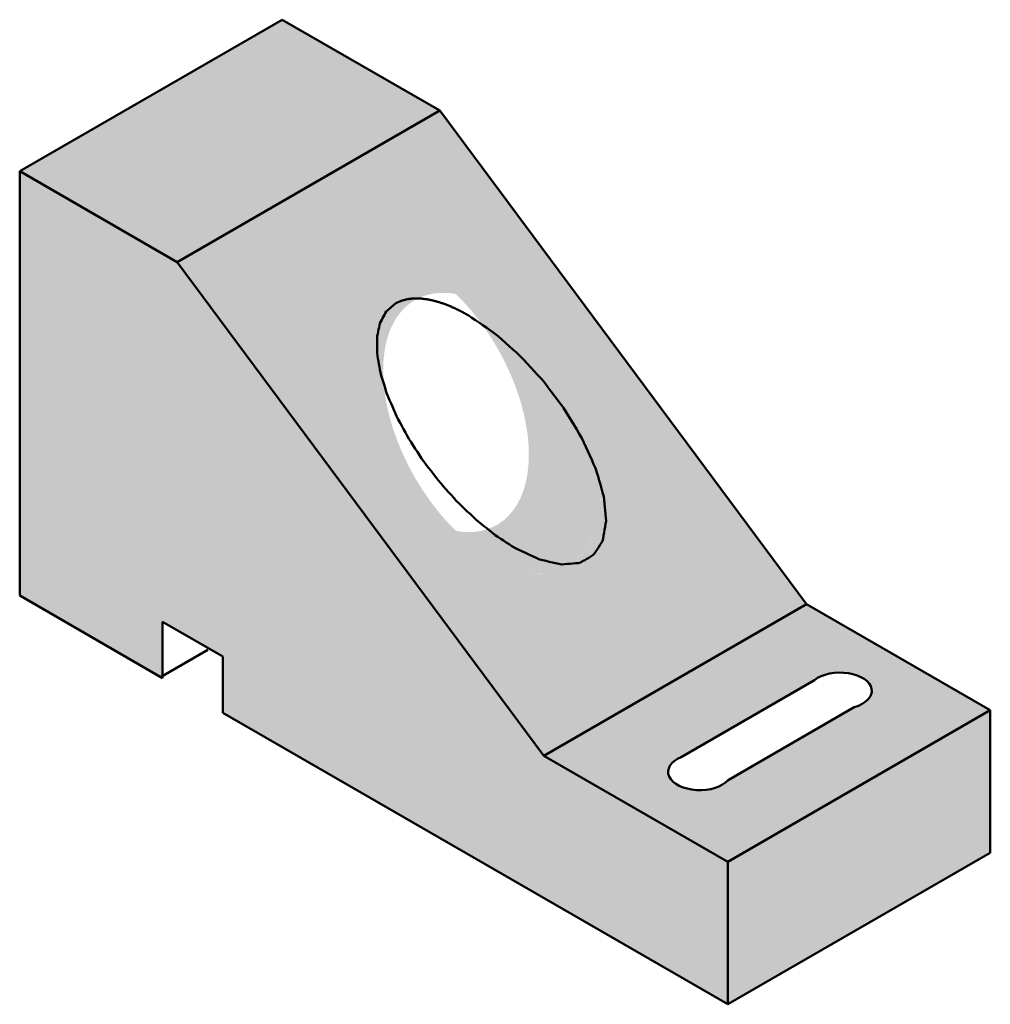
# Model space of a CAD drawing. Units: millimetres. Extents: x 625.96 to 633.96, y 532.78 to 540.9.
import ezdxf

# ---------------------------------------------------------------- set-up
doc = ezdxf.new("R2010")
doc.units = ezdxf.units.MM
doc.header["$MEASUREMENT"] = 0
doc.layers.add('M-HATC', color=7, linetype='Continuous', lineweight=18)
doc.layers.add('M-OUTL', color=7, linetype='Continuous', lineweight=50)

msp = doc.modelspace()

# ---------------------------------------------------------------- hatches: boundary and pattern name
at = {"layer": 'M-HATC'}
h = msp.add_hatch(color=256, dxfattribs=at)
h.dxf.hatch_style = 1
h.set_gradient(color1=(99, 100, 102), tint=1)
h.paths.add_polyline_path([(629.4244087462098, 540.1478741557902), (628.1253706405331, 540.8978741557901), (625.9603071310721, 539.6478741557902), (627.2593452367487, 538.8978741557902)])
h.paths.add_polyline_path([(629.4244087462098, 540.1478741557902), (627.2593452367487, 538.8978741557902), (630.282289748302, 534.8275763282995), (632.4473532577631, 536.0775763282995)])
edge = h.paths.add_edge_path(flags=16)
edge.add_ellipse((629.8533492472558, 537.4877252420449), major_axis=(0.6338907018741607, -1.097930902091765), ratio=0.577350269189629, start_angle=0, end_angle=360)
h.paths.add_polyline_path([(627.2593452367487, 538.8978741557902), (625.9603071310721, 539.6478741557902), (625.9603071310721, 536.1478741557902), (627.1375943885954, 535.4681670407456), (627.1375943885954, 535.9331034747842), (627.6355011647775, 535.6456368635241), (627.6355011647773, 535.1807004294856), (631.7978342049248, 532.7775763282995), (631.7978342049248, 533.9525763282995), (630.282289748302, 534.8275763282995)])
h.paths.add_polyline_path([(633.9628977143859, 535.2025763282995), (632.4473532577631, 536.0775763282995), (630.282289748302, 534.8275763282995), (631.7978342049248, 533.9525763282995)])
edge = h.paths.add_edge_path(flags=16)
edge.add_ellipse((632.7249838710899, 535.3628664376389), major_axis=(-0.2609752309823086, 0), ratio=0.5773502691895677, start_angle=130.8852448293906, end_angle=337.37320687821614, ccw=False)
edge.add_line((632.8416687062745, 535.2280916620266), (631.800863792124, 534.6271826646679))
edge.add_ellipse((631.5674270331846, 534.694550685672), major_axis=(-0.2609752309823086, 0), ratio=0.5773502691895677, start_angle=321.34970944697847, end_angle=523.9022741690201, ccw=False)
edge.add_line((631.4146686328268, 534.8167157956753), (632.5133876936509, 535.451061541206))
h.paths.add_polyline_path([(633.9628977143859, 534.0275763282996), (633.9628977143859, 535.2025763282995), (631.7978342049248, 533.9525763282995), (631.7978342049248, 532.7775763282995)])
h = msp.add_hatch(color=256, dxfattribs=at)
h.dxf.hatch_style = 1
h.set_gradient(color1=(99, 100, 102), tint=1)
edge = h.paths.add_edge_path()
edge.add_ellipse((629.8533492472558, 537.4877252420449), major_axis=(0.6338907018741607, -1.097930902091765), ratio=0.577350269189629, start_angle=309.855821986031, end_angle=524.449523774315)
edge.add_ellipse((629.2617495219952, 537.8292855026767), major_axis=(0.6338907018741607, -1.097930902091765), ratio=0.577350269189629, start_angle=344.4495237743102, end_angle=489.8558219860143, ccw=False)

# ---------------------------------------------------------------- linework, layer by layer
at = {"layer": 'M-OUTL'}
for p, q in [((625.9603071310721, 539.6478741557902), (628.1253706405331, 540.8978741557901)), ((628.1253706405331, 540.8978741557901), (629.4244087462098, 540.1478741557902)), ((627.2593452367487, 538.8978741557902), (629.4244087462098, 540.1478741557902)), ((629.4244087462098, 540.1478741557902), (632.4473532577631, 536.0775763282995)), ((625.9603071310721, 536.1478741557902), (625.9603071310721, 539.6478741557902)), ((625.9603071310721, 539.6478741557902), (627.2593452367487, 538.8978741557902)), ((627.2593452367487, 538.8978741557902), (630.282289748302, 534.8275763282995)), ((625.9603071310721, 536.1478741557902), (627.1375943885954, 535.4681670407456)), ((627.1375943885954, 535.4681670407456), (625.9603071310721, 536.1478741557902)), ((630.282289748302, 534.8275763282995), (632.4473532577631, 536.0775763282995)), ((632.4473532577631, 536.0775763282995), (633.9628977143859, 535.2025763282995)), ((627.1375943885954, 535.4681670407456), (627.1375943885954, 535.9331034747842)), ((627.1375943885954, 535.9331034747842), (627.6355011647775, 535.6456368635241)), ((627.1219216967868, 535.4760275882722), (627.5116331284898, 535.7010275882722)), ((627.6355011647775, 535.6456368635241), (627.6355011647773, 535.1807004294856)), ((631.4146686328268, 534.8167157956753), (632.5133876936518, 535.4510615412065)), ((631.8008637921243, 534.6271826646681), (632.841668706274, 535.2280916620263)), ((631.7978342049248, 532.7775763282995), (627.6355011647773, 535.1807004294856)), ((631.7978342049248, 533.9525763282995), (633.9628977143859, 535.2025763282995)), ((633.9628977143859, 535.2025763282995), (633.9628977143859, 534.0275763282996)), ((630.282289748302, 534.8275763282995), (631.7978342049248, 533.9525763282995)), ((633.9628977143859, 534.0275763282996), (631.7978342049248, 532.7775763282995)), ((631.7978342049248, 533.9525763282995), (631.7978342049248, 532.7775763282995))]:
    msp.add_line(p, q, dxfattribs=at)
for points in [[(630.0416009159691, 536.541821867706), (630.0185722640957, 536.5568658383222), (629.9955436122225, 536.5719098089384), (629.972514960349, 536.5869537795544), (629.9494863084758, 536.6019977501707), (629.9264576566023, 536.6170417207867), (629.9034290047289, 536.632085691403), (629.8803804613445, 536.6476336233994), (629.8572125688939, 536.6662053236779), (629.8340446764432, 536.6847770239561), (629.8108767839924, 536.7033487242346), (629.7877088915416, 536.7219204245129), (629.764540999091, 536.7404921247913), (629.7413731066403, 536.7590638250696), (629.7183524818668, 536.7784935057035), (629.6957000262855, 536.8000681372254), (629.6730475707042, 536.8216427687474), (629.650395115123, 536.8432174002694), (629.6277426595419, 536.8647920317914), (629.6050902039608, 536.8863666633134), (629.5824377483796, 536.9079412948353), (629.5602805281356, 536.9305416161166), (629.5387836216748, 536.9545095237437), (629.5172867152139, 536.978477431371), (629.4957898087531, 537.0024453389979), (629.4742929022923, 537.026413246625), (629.4527959958315, 537.0503811542521), (629.4312990893707, 537.074349061879), (629.4108096159995, 537.0992975362828), (629.3910757174455, 537.1249814357691), (629.3713418188916, 537.1506653352552), (629.3516079203378, 537.1763492347413), (629.331874021784, 537.2020331342273), (629.3121401232299, 537.2277170337135), (629.292406224676, 537.2534009331997), (629.2743299316089, 537.2797921306704), (629.2569166807364, 537.3064662473353), (629.239503429864, 537.333140364), (629.2220901789915, 537.3598144806647), (629.204676928119, 537.3864885973296), (629.1872636772465, 537.4131627139944), (629.1698504263741, 537.4398368306591), (629.1548480703698, 537.4667136281621), (629.140247530177, 537.4936242058047), (629.1256469899841, 537.5205347834471), (629.1110464497912, 537.5474453610898), (629.0964459095985, 537.5743559387323), (629.0818453694056, 537.601266516375), (629.0672448292128, 537.6281770940177), (629.0558695812236, 537.6545636945317), (629.0444943332344, 537.6809502950457), (629.0331190852453, 537.7073368955598), (629.021743837256, 537.7337234960738), (629.0103685892668, 537.7601100965879), (628.9989933412776, 537.786496697102), (628.9881247695085, 537.8127019249434), (628.9802962550594, 537.8378189167489), (628.9724677406102, 537.8629359085543), (628.964639226161, 537.8880529003598), (628.956810711712, 537.9131698921653), (628.9489821972628, 537.9382868839708), (628.9411536828136, 537.9634038757763), (628.9344017259104, 537.9879553350867), (628.9303411628727, 538.0110929631594), (628.926280599835, 538.034230591232), (628.9222200367973, 538.0573682193047), (628.9181594737597, 538.0805058473774), (628.9140989107218, 538.1036434754502), (628.9100383476842, 538.1267811035228), (628.9076417966398, 538.1487902233227), (628.9074639282533, 538.1692946654254), (628.907286059867, 538.1897991075283), (628.9071081914807, 538.2103035496311), (628.9069303230941, 538.2308079917339), (628.9067524547077, 538.2513124338366), (628.9065745863212, 538.2718168759394), (628.908618272706, 538.2904855467647), (628.9123281251692, 538.307777389132), (628.9160379776324, 538.3250692314994), (628.9197478300955, 538.3423610738668), (628.9234576825589, 538.359652916234), (628.927167535022, 538.3769447586013), (628.9308773874852, 538.3942366009685), (628.9372893027884, 538.4088847062098), (628.9447820432277, 538.4224753166005), (628.9522747836671, 538.4360659269912), (628.9597675241063, 538.4496565373819), (628.9672602645456, 538.4632471477726), (628.9747530049849, 538.4768377581632), (628.9822457454242, 538.4904283685539), (628.9927994787729, 538.5005173147089), (629.0038633776065, 538.5100226501577), (629.01492727644, 538.5195279856067), (629.0259911752736, 538.5290333210557), (629.0370550741072, 538.5385386565046), (629.0481189729406, 538.5480439919537), (629.0591828717743, 538.5575493274026)], [(629.0591828717743, 538.5575493274026), (629.0636131434885, 538.5597600192831), (629.0680434152029, 538.5619707111636), (629.072473686917, 538.5641814030441), (629.0769039586312, 538.5663920949247), (629.0813342303455, 538.5686027868053), (629.0857645020596, 538.5708134786857), (629.0902446135747, 538.5729539225624), (629.0950237638945, 538.5746728784162), (629.0998029142143, 538.5763918342698), (629.1045820645342, 538.5781107901236), (629.109361214854, 538.5798297459773), (629.1141403651739, 538.5815487018313), (629.1189195154935, 538.5832676576849), (629.1237940491363, 538.5848445722536), (629.1289070410864, 538.5860663836094), (629.134020033037, 538.5872881949654), (629.1391330249872, 538.5885100063213), (629.1442460169376, 538.5897318176771), (629.1493590088879, 538.5909536290332), (629.1544720008382, 538.5921754403892), (629.1597211731884, 538.5931825422729), (629.165151919405, 538.5939033648604), (629.1705826656214, 538.5946241874481), (629.1760134118381, 538.5953450100355), (629.1814441580545, 538.596065832623), (629.1868749042711, 538.5967866552106), (629.1923056504876, 538.5975074777982), (629.1979082064925, 538.597940725104), (629.2036396198386, 538.5981582909487), (629.2093710331847, 538.5983758567932), (629.2151024465308, 538.5985934226379), (629.2208338598766, 538.5988109884825), (629.2265652732226, 538.5990285543272), (629.2322966865687, 538.5992461201718), (629.238229981331, 538.5991037279553), (629.2442440286598, 538.5988173525142), (629.2502580759883, 538.5985309770734), (629.256272123317, 538.5982446016324), (629.2622861706457, 538.5979582261914), (629.2683002179743, 538.5976718507505), (629.2743142653029, 538.5973854753096), (629.2805543511158, 538.5966679225179), (629.2868321100091, 538.5958785068347), (629.2931098689027, 538.5950890911512), (629.299387627796, 538.5942996754677), (629.3056653866894, 538.5935102597844), (629.3119431455827, 538.5927208441009), (629.3182209044763, 538.5919314284176), (629.3247426227825, 538.5906414562855), (629.3312643410887, 538.5893514841534), (629.337786059395, 538.5880615120213), (629.3443077777011, 538.5867715398894), (629.3508294960072, 538.5854815677573), (629.3573512143134, 538.584191595625), (629.3639048525732, 538.5828306952475), (629.3706500105534, 538.5810442253962), (629.3773951685338, 538.579257755545), (629.384140326514, 538.577471285694), (629.3908854844943, 538.5756848158426), (629.3976306424747, 538.5738983459916), (629.404375800455, 538.5721118761402), (629.4111787346958, 538.570185155768), (629.4181261095879, 538.5679078090927), (629.4250734844799, 538.5656304624175), (629.4320208593718, 538.5633531157423), (629.4389682342639, 538.561075769067), (629.4459156091558, 538.5587984223918), (629.4528629840478, 538.5565210757165), (629.4598876551828, 538.5540364241347), (629.4670153879748, 538.5512753660106), (629.4741431207667, 538.5485143078865), (629.4812708535586, 538.5457532497626), (629.4883985863506, 538.5429921916385), (629.4955263191426, 538.5402311335145), (629.5026540519347, 538.5374700753904), (629.5098720312498, 538.5344375749014), (629.5171576954575, 538.531201492639), (629.524443359665, 538.5279654103762), (629.5317290238726, 538.5247293281138), (629.5390146880801, 538.521493245851), (629.5463003522877, 538.5182571635887), (629.5535860164953, 538.515021081326), (629.5609681150033, 538.5114529689017), (629.5683887872314, 538.5077520444127), (629.5758094594598, 538.5040511199236), (629.5832301316879, 538.5003501954346), (629.5906508039161, 538.4966492709456), (629.5980714761444, 538.4929483464566), (629.6054921483726, 538.4892474219675), (629.6130085290353, 538.4851580422653), (629.6205408611037, 538.4810039200274), (629.6280731931723, 538.4768497977896), (629.635605525241, 538.4726956755518), (629.6431378573093, 538.468541553314), (629.6506701893779, 538.4643874310761), (629.6582025214465, 538.4602333088383)], [(629.6582025214465, 538.4602333088383), (629.6889707599827, 538.4393667454568), (629.7197389985191, 538.4185001820753), (629.7505072370553, 538.3976336186939), (629.7812754755917, 538.3767670553124), (629.8120437141279, 538.3559004919309), (629.8428119526642, 538.3350339285494), (629.8735600468123, 538.3133147880753), (629.9041872746313, 538.2864801850449), (629.9348145024502, 538.2596455820146), (629.9654417302693, 538.232810978984), (629.9960689580882, 538.2059763759538), (630.0266961859074, 538.1791417729233), (630.0573234137264, 538.152307169893), (630.0874715593145, 538.1241518695481), (630.1164219993253, 538.0926948259163), (630.1453724393361, 538.0612377822846), (630.1743228793468, 538.0297807386527), (630.2032733193577, 537.998323695021), (630.2322237593686, 537.9668666513894), (630.2611741993793, 537.9354096077576), (630.2887838606372, 537.9026475413771), (630.3146058168911, 537.8681454446648), (630.3404277731449, 537.8336433479525), (630.3662497293989, 537.7991412512401), (630.3920716856528, 537.764639154528), (630.4178936419066, 537.7301370578156), (630.4437155981605, 537.6956349611035), (630.4670099518621, 537.6603814507436), (630.4884086036495, 537.6245643801481), (630.5098072554368, 537.5887473095527), (630.531205907224, 537.5529302389574), (630.5526045590116, 537.5171131683619), (630.5740032107987, 537.4812960977664), (630.595401862586, 537.445479027171), (630.6128745699305, 537.4100055591439), (630.6287768994976, 537.374669532144), (630.6446792290649, 537.339333505144), (630.6605815586319, 537.3039974781443), (630.6764838881991, 537.2686614511445), (630.6923862177662, 537.2333254241445), (630.7082885473334, 537.1979893971447), (630.7187962499631, 537.164584461179), (630.7284048481033, 537.1315013737188), (630.7380134462435, 537.0984182862586), (630.7476220443835, 537.0653351987985), (630.7572306425238, 537.0322521113384), (630.766839240664, 536.9991690238783), (630.7764478388041, 536.9660859364182), (630.7792808902846, 536.936914712646), (630.7821139417647, 536.9077434888737), (630.7849469932452, 536.8785722651015), (630.7877800447257, 536.8494010413293), (630.7906130962059, 536.8202298175571), (630.7934461476862, 536.7910585937847), (630.7952909694964, 536.7626551743921), (630.7912064132862, 536.7388585812761), (630.7871218570758, 536.7150619881601), (630.7830373008654, 536.6912653950443), (630.7789527446549, 536.6674688019283), (630.7748681884445, 536.6436722088123), (630.7707836322342, 536.6198756156965), (630.7647811357418, 536.5979555629237), (630.7539837885447, 536.5807268610089), (630.7431864413473, 536.563498159094), (630.7323890941504, 536.5462694571792), (630.7215917469532, 536.5290407552642), (630.7107943997561, 536.5118120533493), (630.6999970525588, 536.4945833514345), (630.6865548338278, 536.4805397110578), (630.669586119718, 536.4707428193987), (630.6526174056083, 536.4609459277398), (630.6356486914985, 536.4511490360806), (630.6186799773889, 536.4413521444216), (630.6017112632791, 536.4315552527625), (630.5847425491695, 536.4217583611035), (630.5647335580701, 536.4164889364799), (630.5424443592284, 536.4146151121327), (630.5201551603869, 536.4127412877856), (630.4978659615452, 536.4108674634384), (630.4755767627037, 536.4089936390912), (630.4532875638622, 536.407119814744), (630.4309983650205, 536.4052459903969), (630.4057071581573, 536.4090986151134), (630.3792151480853, 536.4152418194553), (630.3527231380135, 536.4213850237973), (630.3262311279414, 536.4275282281392), (630.2997391178694, 536.4336714324811), (630.2732471077976, 536.4398146368229), (630.2467550977256, 536.4459578411648), (630.217799323747, 536.4587087450253), (630.1884329224508, 536.4725609321387), (630.1590665211545, 536.4864131192522), (630.1297001198581, 536.5002653063656), (630.1003337185618, 536.5141174934791), (630.0709673172654, 536.5279696805925), (630.0416009159691, 536.541821867706)]]:
    msp.add_lwpolyline(points, dxfattribs=at)
for centre, start_param, end_param in [((632.7249838710899, 535.3628664376389), 2.034328971165001, 5.657889943892417), ((631.5674270331846, 534.694550685672), 5.337684343673678, 8.96124531639962)]:
    msp.add_ellipse(centre, major_axis=(-0.2609752309823086, 0), ratio=0.5773502691895677, start_param=start_param, end_param=end_param, dxfattribs=at)

doc.saveas('drawing.dxf')
